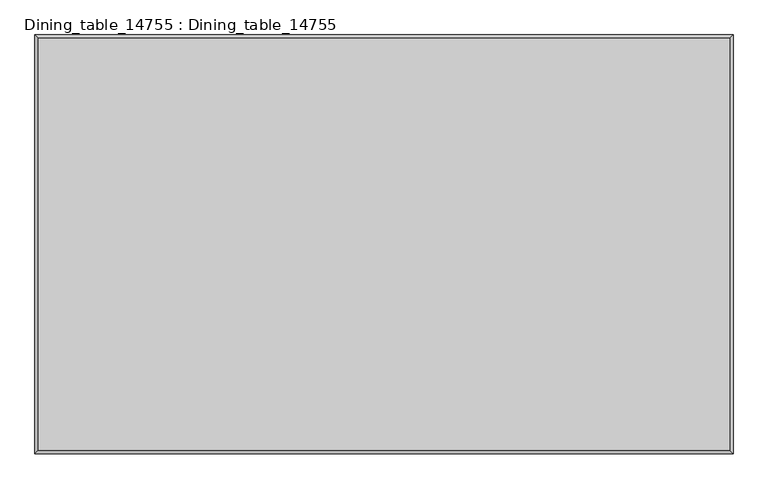
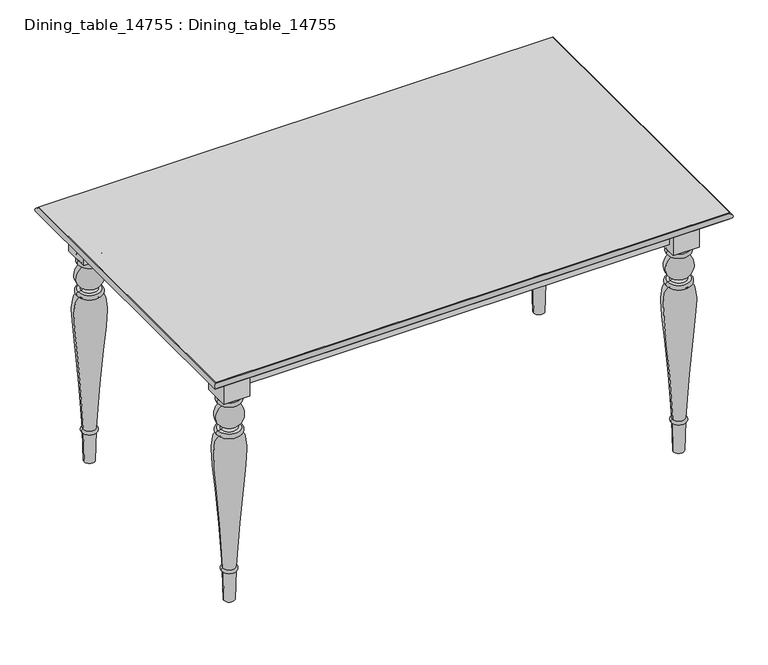
"""IFC4 building model written with IfcOpenShell, lengths in millimetres: furniture geometry, Dining_table_14755 : Dining_table_14755."""

from ifc_helpers import new_model, si_unit, point, frame, origin, place, context, project, spatial, polyline, circle_curve, ellipse_curve, trimmed, outline, extrude, source, transform, mapped, element, save
from ifc_brep_helpers import plane_surface, cylinder_surface, revolved_surface, spline_curve, advanced_brep


def dining_table_14755_dining_table_14755_d89cb775(model_context):
    return source(origin(), model_context, "Body", "SolidModel", [
        extrude(outline(polyline([(137.5044823, 137.5043784), (137.5044823, 62.4956216), (62.4955177, 62.4956216), (62.4955177, 137.5043784), (137.5044823, 137.5043784)])), frame((0.0, 0.0, 630.0), z_axis=(0.0, 0.0, 1.0), x_axis=(1.0, 0.0, 0.0)), (0.0, 0.0, 1.0), 100.0),
        extrude(outline(polyline([(137.5044823, 837.5043784), (137.5044823, 762.4956216), (62.4955177, 762.4956216), (62.4955177, 837.5043784), (137.5044823, 837.5043784)])), frame((0.0, 0.0, 630.0), z_axis=(0.0, 0.0, 1.0), x_axis=(1.0, 0.0, 0.0)), (0.0, 0.0, 1.0), 100.0),
        extrude(outline(polyline([(1437.5044823, 837.5043784), (1437.5044823, 762.4956216), (1362.4955177, 762.4956216), (1362.4955177, 837.5043784), (1437.5044823, 837.5043784)])), frame((0.0, 0.0, 630.0), z_axis=(0.0, 0.0, 1.0), x_axis=(1.0, 0.0, 0.0)), (0.0, 0.0, 1.0), 100.0),
        extrude(outline(polyline([(1437.5044823, 137.5043784), (1437.5044823, 62.4956216), (1362.4955177, 62.4956216), (1362.4955177, 137.5043784), (1437.5044823, 137.5043784)])), frame((0.0, 0.0, 630.0), z_axis=(0.0, 0.0, 1.0), x_axis=(1.0, 0.0, 0.0)), (0.0, 0.0, 1.0), 100.0),
        extrude(outline(polyline([(100.0, 800.0), (100.0, 100.0), (80.0, 100.0), (80.0, 800.0), (100.0, 800.0)])), frame((0.0, 0.0, 655.0), z_axis=(0.0, 0.0, 1.0), x_axis=(1.0, 0.0, 0.0)), (0.0, 0.0, 1.0), 75.0),
        extrude(outline(polyline([(1400.0, 800.0), (100.0, 800.0), (100.0, 820.0), (1400.0, 820.0), (1400.0, 800.0)])), frame((0.0, 0.0, 655.0), z_axis=(0.0, 0.0, 1.0), x_axis=(1.0, 0.0, 0.0)), (0.0, 0.0, 1.0), 75.0),
        extrude(outline(polyline([(1420.0, 800.0), (1420.0, 100.0), (1400.0, 100.0), (1400.0, 800.0), (1420.0, 800.0)])), frame((0.0, 0.0, 655.0), z_axis=(0.0, 0.0, 1.0), x_axis=(1.0, 0.0, 0.0)), (0.0, 0.0, 1.0), 75.0),
        extrude(outline(polyline([(1400.0, 100.0), (1400.0, 80.0), (100.0, 80.0), (100.0, 100.0), (1400.0, 100.0)])), frame((0.0, 0.0, 655.0), z_axis=(0.0, 0.0, 1.0), x_axis=(1.0, 0.0, 0.0)), (0.0, 0.0, 1.0), 75.0),
        advanced_brep(
        [(1492.8253008, 7.1746992, 750.0), (1492.8253008, 892.8253008, 750.0), (7.1746992, 892.8253008, 750.0), (7.1746992, 7.1746992, 750.0), (1492.8253008, 892.8253008, 730.0), (1492.8253008, 7.1746992, 730.0), (7.1746992, 7.1746992, 730.0), (7.1746992, 892.8253008, 730.0), (1492.8253008, 892.8253008, 733.0), (1492.8253008, 7.1746992, 733.0), (1492.8253008, 892.8253008, 747.0), (1492.8253008, 7.1746992, 747.0), (7.1746992, 7.1746992, 733.0), (7.1746992, 7.1746992, 747.0), (7.1746992, 892.8253008, 733.0), (7.1746992, 892.8253008, 747.0)],
        [
            (0, 1),
            (1, 2),
            (2, 3),
            (3, 0),
            (4, 5),
            (5, 6),
            (6, 7),
            (7, 4),
            (8, 9),
            (9, 5),
            (4, 8),
            (8, 10, ellipse_curve(frame((1492.8253008, 892.8253008, 740.0), z_axis=(0.7071067811865475, -0.7071067811865475, 0.0), x_axis=(-0.7071067811865474, -0.7071067811865476, 0.0)), 9.8994949, 7.0)),
            (10, 11),
            (11, 9, ellipse_curve(frame((1492.8253008, 7.1746992, 740.0), z_axis=(0.7071067811865475, 0.7071067811865475, 0.0), x_axis=(0.7071067811865474, -0.7071067811865476, 0.0)), 9.8994949, 7.0)),
            (10, 1),
            (0, 11),
            (9, 12),
            (12, 6),
            (11, 13),
            (13, 12, ellipse_curve(frame((7.1746992, 7.1746992, 740.0), z_axis=(0.7071067811865475, -0.7071067811865475, 0.0), x_axis=(-0.7071067811865476, -0.7071067811865474, 0.0)), 9.8994949, 7.0)),
            (3, 13),
            (12, 14),
            (14, 7),
            (13, 15),
            (15, 14, ellipse_curve(frame((7.1746992, 892.8253008, 740.0), z_axis=(-0.7071067811865475, -0.7071067811865475, 0.0), x_axis=(-0.7071067811865474, 0.7071067811865476, 0.0)), 9.8994949, 7.0)),
            (2, 15),
            (14, 8),
            (15, 10),
        ],
        [
            plane_surface(frame((0.0, 900.0, 750.0), z_axis=(0.0, 0.0, 1.0), x_axis=(-1.0, 0.0, 0.0))),
            plane_surface(frame((0.0, 900.0, 730.0), z_axis=(0.0, 0.0, -1.0), x_axis=(1.0, 0.0, 0.0))),
            plane_surface(frame((1492.8253008, 892.8253008, 730.0), z_axis=(1.0, 0.0, 0.0), x_axis=(0.0, -1.0, 0.0))),
            cylinder_surface(frame((1492.8253008, 900.0, 740.0), z_axis=(0.0, -1.0, 0.0), x_axis=(1.0, 0.0, 0.0)), 7.0),
            plane_surface(frame((1492.8253008, 892.8253008, 747.0), z_axis=(1.0, 0.0, 0.0), x_axis=(0.0, -1.0, 0.0))),
            plane_surface(frame((1492.8253008, 7.1746992, 730.0), z_axis=(0.0, -1.0, 0.0), x_axis=(-1.0, 0.0, 0.0))),
            cylinder_surface(frame((1500.0, 7.1746992, 740.0), z_axis=(-1.0, 0.0, 0.0), x_axis=(0.0, -1.0, 0.0)), 7.0),
            plane_surface(frame((1492.8253008, 7.1746992, 747.0), z_axis=(0.0, -1.0, 0.0), x_axis=(-1.0, 0.0, 0.0))),
            plane_surface(frame((7.1746992, 7.1746992, 730.0), z_axis=(-1.0, 0.0, 0.0), x_axis=(0.0, 1.0, 0.0))),
            cylinder_surface(frame((7.1746992, 0.0, 740.0), z_axis=(0.0, 1.0, 0.0), x_axis=(-1.0, 0.0, 0.0)), 7.0),
            plane_surface(frame((7.1746992, 7.1746992, 747.0), z_axis=(-1.0, 0.0, 0.0), x_axis=(0.0, 1.0, 0.0))),
            plane_surface(frame((7.1746992, 892.8253008, 730.0), z_axis=(0.0, 1.0, 0.0), x_axis=(1.0, 0.0, 0.0))),
            cylinder_surface(frame((0.0, 892.8253008, 740.0), z_axis=(1.0, 0.0, 0.0), x_axis=(0.0, 1.0, 0.0)), 7.0),
            plane_surface(frame((7.1746992, 892.8253008, 747.0), z_axis=(0.0, 1.0, 0.0), x_axis=(1.0, 0.0, 0.0))),
        ],
        [
            (0, [[1, 2, 3, 4]]),
            (1, [[5, 6, 7, 8]]),
            (2, [[9, 10, -5, 11]]),
            (3, [[-9, 12, 13, 14]]),
            (4, [[-13, 15, -1, 16]]),
            (5, [[-10, 17, 18, -6]]),
            (6, [[-14, 19, 20, -17]]),
            (7, [[-16, -4, 21, -19]]),
            (8, [[-18, 22, 23, -7]]),
            (9, [[-20, 24, 25, -22]]),
            (10, [[-21, -3, 26, -24]]),
            (11, [[-11, -8, -23, 27]]),
            (12, [[-12, -27, -25, 28]]),
            (13, [[-15, -28, -26, -2]]),
        ],
    ),
        advanced_brep(
        [(100.0, 100.0, 630.0), (71.6218231, 100.0, 630.0), (128.3781769, 100.0, 630.0), (71.6218231, 100.0, 620.0), (128.3781769, 100.0, 620.0), (71.6218231, 100.0, 607.4843347), (128.3781769, 100.0, 607.4843347), (82.2946134, 100.0, 598.9328748), (117.7053866, 100.0, 598.9328748), (79.4042422, 100.0, 534.8048595), (120.5957578, 100.0, 534.8048595), (77.1750958, 100.0, 526.4855717), (122.8249042, 100.0, 526.4855717), (68.75, 100.0, 525.0), (131.25, 100.0, 525.0), (68.75, 100.0, 513.0), (131.25, 100.0, 513.0), (71.5102534, 100.0, 510.2397466), (128.4897466, 100.0, 510.2397466), (82.3563791, 100.0, 99.9930152), (117.6436209, 100.0, 99.9930152), (82.620575, 100.0, 90.0), (117.379425, 100.0, 90.0), (85.0, 100.0, 0.0), (115.0, 100.0, 0.0), (100.0, 100.0, 0.0)],
        [
            (0, 1),
            (1, 2, circle_curve(frame((100.0, 100.0, 630.0), z_axis=(0.0, 0.0, 1.0), x_axis=(-1.0, 0.0, 0.0)), 28.3781769)),
            (2, 0),
            (2, 1, circle_curve(frame((100.0, 100.0, 630.0), z_axis=(0.0, 0.0, 1.0), x_axis=(-1.0, 0.0, 0.0)), 28.3781769)),
            (1, 3, circle_curve(frame((71.6218231, 100.0, 625.0), z_axis=(0.0, -1.0, 0.0), x_axis=(-1.0, 0.0, 0.0)), 5.0)),
            (3, 4, circle_curve(frame((100.0, 100.0, 620.0), z_axis=(0.0, 0.0, 1.0), x_axis=(-1.0, 0.0, 0.0)), 28.3781769)),
            (4, 2, circle_curve(frame((128.3781769, 100.0, 625.0), z_axis=(0.0, -1.0, 0.0), x_axis=(1.0, 0.0, 0.0)), 5.0)),
            (4, 3, circle_curve(frame((100.0, 100.0, 620.0), z_axis=(0.0, 0.0, 1.0), x_axis=(-1.0, 0.0, 0.0)), 28.3781769)),
            (3, 5, circle_curve(frame((71.6218231, 100.0, 613.7421674), z_axis=(0.0, -1.0, 0.0), x_axis=(-1.0, 0.0, 0.0)), 6.2578326)),
            (5, 6, circle_curve(frame((100.0, 100.0, 607.4843347), z_axis=(0.0, 0.0, 1.0), x_axis=(-1.0, 0.0, 0.0)), 28.3781769)),
            (6, 4, circle_curve(frame((128.3781769, 100.0, 613.7421674), z_axis=(0.0, -1.0, 0.0), x_axis=(1.0, 0.0, 0.0)), 6.2578326)),
            (6, 5, circle_curve(frame((100.0, 100.0, 607.4843347), z_axis=(0.0, 0.0, 1.0), x_axis=(-1.0, 0.0, 0.0)), 28.3781769)),
            (5, 7, circle_curve(frame((71.1386543, 100.0, 595.9454022), z_axis=(0.0, 1.0, 0.0), x_axis=(-1.0, 0.0, 0.0)), 11.5490439)),
            (7, 8, circle_curve(frame((100.0, 100.0, 598.9328748), z_axis=(0.0, 0.0, 1.0), x_axis=(-1.0, 0.0, 0.0)), 17.7053866)),
            (8, 6, circle_curve(frame((128.8613457, 100.0, 595.9454022), z_axis=(0.0, 1.0, 0.0), x_axis=(1.0, 0.0, 0.0)), 11.5490439)),
            (8, 7, circle_curve(frame((100.0, 100.0, 598.9328748), z_axis=(0.0, 0.0, 1.0), x_axis=(-1.0, 0.0, 0.0)), 17.7053866)),
            (7, 9, circle_curve(frame((97.4307139, 100.0, 566.1215172), z_axis=(0.0, -1.0, 0.0), x_axis=(-1.0, 0.0, 0.0)), 36.1342874)),
            (9, 10, circle_curve(frame((100.0, 100.0, 534.8048595), z_axis=(0.0, 0.0, 1.0), x_axis=(-1.0, 0.0, 0.0)), 20.5957578)),
            (10, 8, circle_curve(frame((102.5692861, 100.0, 566.1215172), z_axis=(0.0, -1.0, 0.0), x_axis=(1.0, 0.0, 0.0)), 36.1342874)),
            (10, 9, circle_curve(frame((100.0, 100.0, 534.8048595), z_axis=(0.0, 0.0, 1.0), x_axis=(-1.0, 0.0, 0.0)), 20.5957578)),
            (9, 11, circle_curve(frame((76.3499952, 100.0, 531.1649497), z_axis=(0.0, 1.0, 0.0), x_axis=(-1.0, 0.0, 0.0)), 4.7515649)),
            (11, 12, circle_curve(frame((100.0, 100.0, 526.4855717), z_axis=(0.0, 0.0, 1.0), x_axis=(-1.0, 0.0, 0.0)), 22.8249042)),
            (12, 10, circle_curve(frame((123.6500048, 100.0, 531.1649497), z_axis=(0.0, 1.0, 0.0), x_axis=(1.0, 0.0, 0.0)), 4.7515649)),
            (12, 11, circle_curve(frame((100.0, 100.0, 526.4855717), z_axis=(0.0, 0.0, 1.0), x_axis=(-1.0, 0.0, 0.0)), 22.8249042)),
            (11, 13),
            (13, 14, circle_curve(frame((100.0, 100.0, 525.0), z_axis=(0.0, 0.0, 1.0), x_axis=(-1.0, 0.0, 0.0)), 31.25)),
            (14, 12),
            (14, 13, circle_curve(frame((100.0, 100.0, 525.0), z_axis=(0.0, 0.0, 1.0), x_axis=(-1.0, 0.0, 0.0)), 31.25)),
            (13, 15, circle_curve(frame((68.75, 100.0, 519.0), z_axis=(0.0, -1.0, 0.0), x_axis=(-1.0, 0.0, 0.0)), 6.0)),
            (15, 16, circle_curve(frame((100.0, 100.0, 513.0), z_axis=(0.0, 0.0, 1.0), x_axis=(-1.0, 0.0, 0.0)), 31.25)),
            (16, 14, circle_curve(frame((131.25, 100.0, 519.0), z_axis=(0.0, -1.0, 0.0), x_axis=(1.0, 0.0, 0.0)), 6.0)),
            (16, 15, circle_curve(frame((100.0, 100.0, 513.0), z_axis=(0.0, 0.0, 1.0), x_axis=(-1.0, 0.0, 0.0)), 31.25)),
            (15, 17),
            (17, 18, circle_curve(frame((100.0, 100.0, 510.2397466), z_axis=(0.0, 0.0, 1.0), x_axis=(-1.0, 0.0, 0.0)), 28.4897466)),
            (18, 16),
            (18, 17, circle_curve(frame((100.0, 100.0, 510.2397466), z_axis=(0.0, 0.0, 1.0), x_axis=(-1.0, 0.0, 0.0)), 28.4897466)),
            (17, 19, spline_curve(3, [(71.5102534, 100.0, 510.2397466), (36.079208212, 100.0, 493.717978887), (66.498177461, 100.0, 402.585528177), (82.3563791, 100.0, 99.9930152)], [4, 4], [0.0, 0.4791959451561188])),
            (19, 20, circle_curve(frame((100.0, 100.0, 99.9930152), z_axis=(0.0, 0.0, 1.0), x_axis=(-1.0, 0.0, 0.0)), 17.6436209)),
            (20, 18, spline_curve(3, [(117.6436209, 100.0, 99.9930152), (133.501822539, 100.0, 402.585528177), (163.920791788, 100.0, 493.717978887), (128.4897466, 100.0, 510.2397466)], [4, 4], [0.0, 0.4791959451561188])),
            (20, 19, circle_curve(frame((100.0, 100.0, 99.9930152), z_axis=(0.0, 0.0, 1.0), x_axis=(-1.0, 0.0, 0.0)), 17.6436209)),
            (19, 21, circle_curve(frame((82.620575, 100.0, 95.0), z_axis=(0.0, -1.0, 0.0), x_axis=(-1.0, 0.0, 0.0)), 5.0)),
            (21, 22, circle_curve(frame((100.0, 100.0, 90.0), z_axis=(0.0, 0.0, 1.0), x_axis=(-1.0, 0.0, 0.0)), 17.379425)),
            (22, 20, circle_curve(frame((117.379425, 100.0, 95.0), z_axis=(0.0, -1.0, 0.0), x_axis=(1.0, 0.0, 0.0)), 5.0)),
            (22, 21, circle_curve(frame((100.0, 100.0, 90.0), z_axis=(0.0, 0.0, 1.0), x_axis=(-1.0, 0.0, 0.0)), 17.379425)),
            (21, 23),
            (23, 24, circle_curve(frame((100.0, 100.0, 0.0), z_axis=(0.0, 0.0, 1.0), x_axis=(-1.0, 0.0, 0.0)), 15.0)),
            (24, 22),
            (24, 23, circle_curve(frame((100.0, 100.0, 0.0), z_axis=(0.0, 0.0, 1.0), x_axis=(-1.0, 0.0, 0.0)), 15.0)),
            (23, 25),
            (25, 24),
        ],
        [
            plane_surface(frame((100.0, 100.0, 630.0), z_axis=(0.0, 0.0, 1.0), x_axis=(-1.0, 0.0, 0.0))),
            revolved_surface(trimmed(ellipse_curve(frame((71.6218231, 100.0, 625.0), z_axis=(0.0, 1.0, 0.0), x_axis=(-1.0, 0.0, 0.0)), 5.0, 5.0), [point((71.6218231, 100.0, 620.0))], [point((71.6218231, 100.0, 630.0))], True, "CARTESIAN"), (100.0, 100.0, 950.0), (0.0, 0.0, 1.0)),
            revolved_surface(trimmed(ellipse_curve(frame((71.6218231, 100.0, 613.7421674), z_axis=(0.0, 1.0, 0.0), x_axis=(-1.0, 0.0, 0.0)), 6.2578326, 6.2578326), [point((71.6218231, 100.0, 607.4843347))], [point((71.6218231, 100.0, 620.0))], True, "CARTESIAN"), (100.0, 100.0, 950.0), (0.0, 0.0, 1.0)),
            revolved_surface(trimmed(ellipse_curve(frame((71.1386543, 100.0, 595.9454022), z_axis=(0.0, -1.0, 0.0), x_axis=(-1.0, 0.0, 0.0)), 11.5490439, 11.5490439), [point((82.2946134, 100.0, 598.9328748))], [point((71.6218231, 100.0, 607.4843347))], True, "CARTESIAN"), (100.0, 100.0, 950.0), (0.0, 0.0, 1.0)),
            revolved_surface(trimmed(ellipse_curve(frame((97.4307139, 100.0, 566.1215172), z_axis=(0.0, 1.0, 0.0), x_axis=(-1.0, 0.0, 0.0)), 36.1342874, 36.1342874), [point((79.4042422, 100.0, 534.8048595))], [point((82.2946134, 100.0, 598.9328748))], True, "CARTESIAN"), (100.0, 100.0, 950.0), (0.0, 0.0, 1.0)),
            revolved_surface(trimmed(ellipse_curve(frame((76.3499952, 100.0, 531.1649497), z_axis=(0.0, -1.0, 0.0), x_axis=(-1.0, 0.0, 0.0)), 4.7515649, 4.7515649), [point((77.1750958, 100.0, 526.4855717))], [point((79.4042422, 100.0, 534.8048595))], True, "CARTESIAN"), (100.0, 100.0, 950.0), (0.0, 0.0, 1.0)),
            revolved_surface(polyline([(68.75, 100.0, 525.0), (77.1750958, 100.0, 526.4855717)]), (100.0, 100.0, 950.0), (0.0, 0.0, 1.0)),
            revolved_surface(trimmed(ellipse_curve(frame((68.75, 100.0, 519.0), z_axis=(0.0, 1.0, 0.0), x_axis=(-1.0, 0.0, 0.0)), 6.0, 6.0), [point((68.75, 100.0, 513.0))], [point((68.75, 100.0, 525.0))], True, "CARTESIAN"), (100.0, 100.0, 950.0), (0.0, 0.0, 1.0)),
            revolved_surface(polyline([(71.5102534, 100.0, 510.2397466), (68.75, 100.0, 513.0)]), (100.0, 100.0, 950.0), (0.0, 0.0, 1.0)),
            revolved_surface(spline_curve(3, [(82.3563791, 100.0, 99.9930152), (66.498177461, 100.0, 402.585528177), (36.079208212, 100.0, 493.717978887), (71.5102534, 100.0, 510.2397466)], [4, 4], [0.0, 0.4791959451561188]), (100.0, 100.0, 950.0), (0.0, 0.0, 1.0)),
            revolved_surface(trimmed(ellipse_curve(frame((82.620575, 100.0, 95.0), z_axis=(0.0, 1.0, 0.0), x_axis=(-1.0, 0.0, 0.0)), 5.0, 5.0), [point((82.620575, 100.0, 90.0))], [point((82.3563791, 100.0, 99.9930152))], True, "CARTESIAN"), (100.0, 100.0, 950.0), (0.0, 0.0, 1.0)),
            revolved_surface(polyline([(85.0, 100.0, 0.0), (82.620575, 100.0, 90.0)]), (100.0, 100.0, 950.0), (0.0, 0.0, 1.0)),
            plane_surface(frame((100.0, 100.0, 0.0), z_axis=(0.0, 0.0, -1.0), x_axis=(-1.0, 0.0, 0.0))),
        ],
        [
            (0, [[1, 2, 3]]),
            (0, [[-3, 4, -1]]),
            (1, [[-2, 5, 6, 7]]),
            (1, [[-4, -7, 8, -5]]),
            (2, [[-6, 9, 10, 11]]),
            (2, [[-8, -11, 12, -9]]),
            (3, [[-10, 13, 14, 15]]),
            (3, [[-12, -15, 16, -13]]),
            (4, [[-14, 17, 18, 19]]),
            (4, [[-16, -19, 20, -17]]),
            (5, [[-18, 21, 22, 23]]),
            (5, [[-20, -23, 24, -21]]),
            (6, [[-22, 25, 26, 27]]),
            (6, [[-24, -27, 28, -25]]),
            (7, [[-26, 29, 30, 31]]),
            (7, [[-28, -31, 32, -29]]),
            (8, [[-30, 33, 34, 35]]),
            (8, [[-32, -35, 36, -33]]),
            (9, [[-34, 37, 38, 39]]),
            (9, [[-36, -39, 40, -37]]),
            (10, [[-38, 41, 42, 43]]),
            (10, [[-40, -43, 44, -41]]),
            (11, [[-42, 45, 46, 47]]),
            (11, [[-44, -47, 48, -45]]),
            (12, [[-46, 49, 50]]),
            (12, [[-48, -50, -49]]),
        ],
    ),
        advanced_brep(
        [(100.0, 800.0, 630.0), (71.6218231, 800.0, 630.0), (128.3781769, 800.0, 630.0), (71.6218231, 800.0, 620.0), (128.3781769, 800.0, 620.0), (71.6218231, 800.0, 607.4843347), (128.3781769, 800.0, 607.4843347), (82.2946134, 800.0, 598.9328748), (117.7053866, 800.0, 598.9328748), (79.4042422, 800.0, 534.8048595), (120.5957578, 800.0, 534.8048595), (77.1750958, 800.0, 526.4855717), (122.8249042, 800.0, 526.4855717), (68.75, 800.0, 525.0), (131.25, 800.0, 525.0), (68.75, 800.0, 513.0), (131.25, 800.0, 513.0), (71.5102534, 800.0, 510.2397466), (128.4897466, 800.0, 510.2397466), (82.3563791, 800.0, 99.9930152), (117.6436209, 800.0, 99.9930152), (82.620575, 800.0, 90.0), (117.379425, 800.0, 90.0), (85.0, 800.0, 0.0), (115.0, 800.0, 0.0), (100.0, 800.0, 0.0)],
        [
            (0, 1),
            (1, 2, circle_curve(frame((100.0, 800.0, 630.0), z_axis=(0.0, 0.0, 1.0), x_axis=(-1.0, 0.0, 0.0)), 28.3781769)),
            (2, 0),
            (2, 1, circle_curve(frame((100.0, 800.0, 630.0), z_axis=(0.0, 0.0, 1.0), x_axis=(-1.0, 0.0, 0.0)), 28.3781769)),
            (1, 3, circle_curve(frame((71.6218231, 800.0, 625.0), z_axis=(0.0, -1.0, 0.0), x_axis=(-1.0, 0.0, 0.0)), 5.0)),
            (3, 4, circle_curve(frame((100.0, 800.0, 620.0), z_axis=(0.0, 0.0, 1.0), x_axis=(-1.0, 0.0, 0.0)), 28.3781769)),
            (4, 2, circle_curve(frame((128.3781769, 800.0, 625.0), z_axis=(0.0, -1.0, 0.0), x_axis=(1.0, 0.0, 0.0)), 5.0)),
            (4, 3, circle_curve(frame((100.0, 800.0, 620.0), z_axis=(0.0, 0.0, 1.0), x_axis=(-1.0, 0.0, 0.0)), 28.3781769)),
            (3, 5, circle_curve(frame((71.6218231, 800.0, 613.7421674), z_axis=(0.0, -1.0, 0.0), x_axis=(-1.0, 0.0, 0.0)), 6.2578326)),
            (5, 6, circle_curve(frame((100.0, 800.0, 607.4843347), z_axis=(0.0, 0.0, 1.0), x_axis=(-1.0, 0.0, 0.0)), 28.3781769)),
            (6, 4, circle_curve(frame((128.3781769, 800.0, 613.7421674), z_axis=(0.0, -1.0, 0.0), x_axis=(1.0, 0.0, 0.0)), 6.2578326)),
            (6, 5, circle_curve(frame((100.0, 800.0, 607.4843347), z_axis=(0.0, 0.0, 1.0), x_axis=(-1.0, 0.0, 0.0)), 28.3781769)),
            (5, 7, circle_curve(frame((71.1386543, 800.0, 595.9454022), z_axis=(0.0, 1.0, 0.0), x_axis=(-1.0, 0.0, 0.0)), 11.5490439)),
            (7, 8, circle_curve(frame((100.0, 800.0, 598.9328748), z_axis=(0.0, 0.0, 1.0), x_axis=(-1.0, 0.0, 0.0)), 17.7053866)),
            (8, 6, circle_curve(frame((128.8613457, 800.0, 595.9454022), z_axis=(0.0, 1.0, 0.0), x_axis=(1.0, 0.0, 0.0)), 11.5490439)),
            (8, 7, circle_curve(frame((100.0, 800.0, 598.9328748), z_axis=(0.0, 0.0, 1.0), x_axis=(-1.0, 0.0, 0.0)), 17.7053866)),
            (7, 9, circle_curve(frame((97.4307139, 800.0, 566.1215172), z_axis=(0.0, -1.0, 0.0), x_axis=(-1.0, 0.0, 0.0)), 36.1342874)),
            (9, 10, circle_curve(frame((100.0, 800.0, 534.8048595), z_axis=(0.0, 0.0, 1.0), x_axis=(-1.0, 0.0, 0.0)), 20.5957578)),
            (10, 8, circle_curve(frame((102.5692861, 800.0, 566.1215172), z_axis=(0.0, -1.0, 0.0), x_axis=(1.0, 0.0, 0.0)), 36.1342874)),
            (10, 9, circle_curve(frame((100.0, 800.0, 534.8048595), z_axis=(0.0, 0.0, 1.0), x_axis=(-1.0, 0.0, 0.0)), 20.5957578)),
            (9, 11, circle_curve(frame((76.3499952, 800.0, 531.1649497), z_axis=(0.0, 1.0, 0.0), x_axis=(-1.0, 0.0, 0.0)), 4.7515649)),
            (11, 12, circle_curve(frame((100.0, 800.0, 526.4855717), z_axis=(0.0, 0.0, 1.0), x_axis=(-1.0, 0.0, 0.0)), 22.8249042)),
            (12, 10, circle_curve(frame((123.6500048, 800.0, 531.1649497), z_axis=(0.0, 1.0, 0.0), x_axis=(1.0, 0.0, 0.0)), 4.7515649)),
            (12, 11, circle_curve(frame((100.0, 800.0, 526.4855717), z_axis=(0.0, 0.0, 1.0), x_axis=(-1.0, 0.0, 0.0)), 22.8249042)),
            (11, 13),
            (13, 14, circle_curve(frame((100.0, 800.0, 525.0), z_axis=(0.0, 0.0, 1.0), x_axis=(-1.0, 0.0, 0.0)), 31.25)),
            (14, 12),
            (14, 13, circle_curve(frame((100.0, 800.0, 525.0), z_axis=(0.0, 0.0, 1.0), x_axis=(-1.0, 0.0, 0.0)), 31.25)),
            (13, 15, circle_curve(frame((68.75, 800.0, 519.0), z_axis=(0.0, -1.0, 0.0), x_axis=(-1.0, 0.0, 0.0)), 6.0)),
            (15, 16, circle_curve(frame((100.0, 800.0, 513.0), z_axis=(0.0, 0.0, 1.0), x_axis=(-1.0, 0.0, 0.0)), 31.25)),
            (16, 14, circle_curve(frame((131.25, 800.0, 519.0), z_axis=(0.0, -1.0, 0.0), x_axis=(1.0, 0.0, 0.0)), 6.0)),
            (16, 15, circle_curve(frame((100.0, 800.0, 513.0), z_axis=(0.0, 0.0, 1.0), x_axis=(-1.0, 0.0, 0.0)), 31.25)),
            (15, 17),
            (17, 18, circle_curve(frame((100.0, 800.0, 510.2397466), z_axis=(0.0, 0.0, 1.0), x_axis=(-1.0, 0.0, 0.0)), 28.4897466)),
            (18, 16),
            (18, 17, circle_curve(frame((100.0, 800.0, 510.2397466), z_axis=(0.0, 0.0, 1.0), x_axis=(-1.0, 0.0, 0.0)), 28.4897466)),
            (17, 19, spline_curve(3, [(71.5102534, 800.0, 510.2397466), (36.079208212, 800.0, 493.717978887), (66.498177461, 800.0, 402.585528177), (82.3563791, 800.0, 99.9930152)], [4, 4], [0.0, 0.4791959451561188])),
            (19, 20, circle_curve(frame((100.0, 800.0, 99.9930152), z_axis=(0.0, 0.0, 1.0), x_axis=(-1.0, 0.0, 0.0)), 17.6436209)),
            (20, 18, spline_curve(3, [(117.6436209, 800.0, 99.9930152), (133.501822539, 800.0, 402.585528177), (163.920791788, 800.0, 493.717978887), (128.4897466, 800.0, 510.2397466)], [4, 4], [0.0, 0.4791959451561188])),
            (20, 19, circle_curve(frame((100.0, 800.0, 99.9930152), z_axis=(0.0, 0.0, 1.0), x_axis=(-1.0, 0.0, 0.0)), 17.6436209)),
            (19, 21, circle_curve(frame((82.620575, 800.0, 95.0), z_axis=(0.0, -1.0, 0.0), x_axis=(-1.0, 0.0, 0.0)), 5.0)),
            (21, 22, circle_curve(frame((100.0, 800.0, 90.0), z_axis=(0.0, 0.0, 1.0), x_axis=(-1.0, 0.0, 0.0)), 17.379425)),
            (22, 20, circle_curve(frame((117.379425, 800.0, 95.0), z_axis=(0.0, -1.0, 0.0), x_axis=(1.0, 0.0, 0.0)), 5.0)),
            (22, 21, circle_curve(frame((100.0, 800.0, 90.0), z_axis=(0.0, 0.0, 1.0), x_axis=(-1.0, 0.0, 0.0)), 17.379425)),
            (21, 23),
            (23, 24, circle_curve(frame((100.0, 800.0, 0.0), z_axis=(0.0, 0.0, 1.0), x_axis=(-1.0, 0.0, 0.0)), 15.0)),
            (24, 22),
            (24, 23, circle_curve(frame((100.0, 800.0, 0.0), z_axis=(0.0, 0.0, 1.0), x_axis=(-1.0, 0.0, 0.0)), 15.0)),
            (23, 25),
            (25, 24),
        ],
        [
            plane_surface(frame((100.0, 800.0, 630.0), z_axis=(0.0, 0.0, 1.0), x_axis=(-1.0, 0.0, 0.0))),
            revolved_surface(trimmed(ellipse_curve(frame((71.6218231, 800.0, 625.0), z_axis=(0.0, 1.0, 0.0), x_axis=(-1.0, 0.0, 0.0)), 5.0, 5.0), [point((71.6218231, 800.0, 620.0))], [point((71.6218231, 800.0, 630.0))], True, "CARTESIAN"), (100.0, 800.0, 950.0), (0.0, 0.0, 1.0)),
            revolved_surface(trimmed(ellipse_curve(frame((71.6218231, 800.0, 613.7421674), z_axis=(0.0, 1.0, 0.0), x_axis=(-1.0, 0.0, 0.0)), 6.2578326, 6.2578326), [point((71.6218231, 800.0, 607.4843347))], [point((71.6218231, 800.0, 620.0))], True, "CARTESIAN"), (100.0, 800.0, 950.0), (0.0, 0.0, 1.0)),
            revolved_surface(trimmed(ellipse_curve(frame((71.1386543, 800.0, 595.9454022), z_axis=(0.0, -1.0, 0.0), x_axis=(-1.0, 0.0, 0.0)), 11.5490439, 11.5490439), [point((82.2946134, 800.0, 598.9328748))], [point((71.6218231, 800.0, 607.4843347))], True, "CARTESIAN"), (100.0, 800.0, 950.0), (0.0, 0.0, 1.0)),
            revolved_surface(trimmed(ellipse_curve(frame((97.4307139, 800.0, 566.1215172), z_axis=(0.0, 1.0, 0.0), x_axis=(-1.0, 0.0, 0.0)), 36.1342874, 36.1342874), [point((79.4042422, 800.0, 534.8048595))], [point((82.2946134, 800.0, 598.9328748))], True, "CARTESIAN"), (100.0, 800.0, 950.0), (0.0, 0.0, 1.0)),
            revolved_surface(trimmed(ellipse_curve(frame((76.3499952, 800.0, 531.1649497), z_axis=(0.0, -1.0, 0.0), x_axis=(-1.0, 0.0, 0.0)), 4.7515649, 4.7515649), [point((77.1750958, 800.0, 526.4855717))], [point((79.4042422, 800.0, 534.8048595))], True, "CARTESIAN"), (100.0, 800.0, 950.0), (0.0, 0.0, 1.0)),
            revolved_surface(polyline([(68.75, 800.0, 525.0), (77.1750958, 800.0, 526.4855717)]), (100.0, 800.0, 950.0), (0.0, 0.0, 1.0)),
            revolved_surface(trimmed(ellipse_curve(frame((68.75, 800.0, 519.0), z_axis=(0.0, 1.0, 0.0), x_axis=(-1.0, 0.0, 0.0)), 6.0, 6.0), [point((68.75, 800.0, 513.0))], [point((68.75, 800.0, 525.0))], True, "CARTESIAN"), (100.0, 800.0, 950.0), (0.0, 0.0, 1.0)),
            revolved_surface(polyline([(71.5102534, 800.0, 510.2397466), (68.75, 800.0, 513.0)]), (100.0, 800.0, 950.0), (0.0, 0.0, 1.0)),
            revolved_surface(spline_curve(3, [(82.3563791, 800.0, 99.9930152), (66.498177461, 800.0, 402.585528177), (36.079208212, 800.0, 493.717978887), (71.5102534, 800.0, 510.2397466)], [4, 4], [0.0, 0.4791959451561188]), (100.0, 800.0, 950.0), (0.0, 0.0, 1.0)),
            revolved_surface(trimmed(ellipse_curve(frame((82.620575, 800.0, 95.0), z_axis=(0.0, 1.0, 0.0), x_axis=(-1.0, 0.0, 0.0)), 5.0, 5.0), [point((82.620575, 800.0, 90.0))], [point((82.3563791, 800.0, 99.9930152))], True, "CARTESIAN"), (100.0, 800.0, 950.0), (0.0, 0.0, 1.0)),
            revolved_surface(polyline([(85.0, 800.0, 0.0), (82.620575, 800.0, 90.0)]), (100.0, 800.0, 950.0), (0.0, 0.0, 1.0)),
            plane_surface(frame((100.0, 800.0, 0.0), z_axis=(0.0, 0.0, -1.0), x_axis=(-1.0, 0.0, 0.0))),
        ],
        [
            (0, [[1, 2, 3]]),
            (0, [[-3, 4, -1]]),
            (1, [[-2, 5, 6, 7]]),
            (1, [[-4, -7, 8, -5]]),
            (2, [[-6, 9, 10, 11]]),
            (2, [[-8, -11, 12, -9]]),
            (3, [[-10, 13, 14, 15]]),
            (3, [[-12, -15, 16, -13]]),
            (4, [[-14, 17, 18, 19]]),
            (4, [[-16, -19, 20, -17]]),
            (5, [[-18, 21, 22, 23]]),
            (5, [[-20, -23, 24, -21]]),
            (6, [[-22, 25, 26, 27]]),
            (6, [[-24, -27, 28, -25]]),
            (7, [[-26, 29, 30, 31]]),
            (7, [[-28, -31, 32, -29]]),
            (8, [[-30, 33, 34, 35]]),
            (8, [[-32, -35, 36, -33]]),
            (9, [[-34, 37, 38, 39]]),
            (9, [[-36, -39, 40, -37]]),
            (10, [[-38, 41, 42, 43]]),
            (10, [[-40, -43, 44, -41]]),
            (11, [[-42, 45, 46, 47]]),
            (11, [[-44, -47, 48, -45]]),
            (12, [[-46, 49, 50]]),
            (12, [[-48, -50, -49]]),
        ],
    ),
        advanced_brep(
        [(1400.0, 800.0, 630.0), (1371.6218231, 800.0, 630.0), (1428.3781769, 800.0, 630.0), (1371.6218231, 800.0, 620.0), (1428.3781769, 800.0, 620.0), (1371.6218231, 800.0, 607.4843347), (1428.3781769, 800.0, 607.4843347), (1382.2946134, 800.0, 598.9328748), (1417.7053866, 800.0, 598.9328748), (1379.4042422, 800.0, 534.8048595), (1420.5957578, 800.0, 534.8048595), (1377.1750958, 800.0, 526.4855717), (1422.8249042, 800.0, 526.4855717), (1368.75, 800.0, 525.0), (1431.25, 800.0, 525.0), (1368.75, 800.0, 513.0), (1431.25, 800.0, 513.0), (1371.5102534, 800.0, 510.2397466), (1428.4897466, 800.0, 510.2397466), (1382.3563791, 800.0, 99.9930152), (1417.6436209, 800.0, 99.9930152), (1382.620575, 800.0, 90.0), (1417.379425, 800.0, 90.0), (1385.0, 800.0, 0.0), (1415.0, 800.0, 0.0), (1400.0, 800.0, 0.0)],
        [
            (0, 1),
            (1, 2, circle_curve(frame((1400.0, 800.0, 630.0), z_axis=(0.0, 0.0, 1.0), x_axis=(-1.0, 0.0, 0.0)), 28.3781769)),
            (2, 0),
            (2, 1, circle_curve(frame((1400.0, 800.0, 630.0), z_axis=(0.0, 0.0, 1.0), x_axis=(-1.0, 0.0, 0.0)), 28.3781769)),
            (1, 3, circle_curve(frame((1371.6218231, 800.0, 625.0), z_axis=(0.0, -1.0, 0.0), x_axis=(-1.0, 0.0, 0.0)), 5.0)),
            (3, 4, circle_curve(frame((1400.0, 800.0, 620.0), z_axis=(0.0, 0.0, 1.0), x_axis=(-1.0, 0.0, 0.0)), 28.3781769)),
            (4, 2, circle_curve(frame((1428.3781769, 800.0, 625.0), z_axis=(0.0, -1.0, 0.0), x_axis=(1.0, 0.0, 0.0)), 5.0)),
            (4, 3, circle_curve(frame((1400.0, 800.0, 620.0), z_axis=(0.0, 0.0, 1.0), x_axis=(-1.0, 0.0, 0.0)), 28.3781769)),
            (3, 5, circle_curve(frame((1371.6218231, 800.0, 613.7421674), z_axis=(0.0, -1.0, 0.0), x_axis=(-1.0, 0.0, 0.0)), 6.2578326)),
            (5, 6, circle_curve(frame((1400.0, 800.0, 607.4843347), z_axis=(0.0, 0.0, 1.0), x_axis=(-1.0, 0.0, 0.0)), 28.3781769)),
            (6, 4, circle_curve(frame((1428.3781769, 800.0, 613.7421674), z_axis=(0.0, -1.0, 0.0), x_axis=(1.0, 0.0, 0.0)), 6.2578326)),
            (6, 5, circle_curve(frame((1400.0, 800.0, 607.4843347), z_axis=(0.0, 0.0, 1.0), x_axis=(-1.0, 0.0, 0.0)), 28.3781769)),
            (5, 7, circle_curve(frame((1371.1386543, 800.0, 595.9454022), z_axis=(0.0, 1.0, 0.0), x_axis=(-1.0, 0.0, 0.0)), 11.5490439)),
            (7, 8, circle_curve(frame((1400.0, 800.0, 598.9328748), z_axis=(0.0, 0.0, 1.0), x_axis=(-1.0, 0.0, 0.0)), 17.7053866)),
            (8, 6, circle_curve(frame((1428.8613457, 800.0, 595.9454022), z_axis=(0.0, 1.0, 0.0), x_axis=(1.0, 0.0, 0.0)), 11.5490439)),
            (8, 7, circle_curve(frame((1400.0, 800.0, 598.9328748), z_axis=(0.0, 0.0, 1.0), x_axis=(-1.0, 0.0, 0.0)), 17.7053866)),
            (7, 9, circle_curve(frame((1397.4307139, 800.0, 566.1215172), z_axis=(0.0, -1.0, 0.0), x_axis=(-1.0, 0.0, 0.0)), 36.1342874)),
            (9, 10, circle_curve(frame((1400.0, 800.0, 534.8048595), z_axis=(0.0, 0.0, 1.0), x_axis=(-1.0, 0.0, 0.0)), 20.5957578)),
            (10, 8, circle_curve(frame((1402.5692861, 800.0, 566.1215172), z_axis=(0.0, -1.0, 0.0), x_axis=(1.0, 0.0, 0.0)), 36.1342874)),
            (10, 9, circle_curve(frame((1400.0, 800.0, 534.8048595), z_axis=(0.0, 0.0, 1.0), x_axis=(-1.0, 0.0, 0.0)), 20.5957578)),
            (9, 11, circle_curve(frame((1376.3499952, 800.0, 531.1649497), z_axis=(0.0, 1.0, 0.0), x_axis=(-1.0, 0.0, 0.0)), 4.7515649)),
            (11, 12, circle_curve(frame((1400.0, 800.0, 526.4855717), z_axis=(0.0, 0.0, 1.0), x_axis=(-1.0, 0.0, 0.0)), 22.8249042)),
            (12, 10, circle_curve(frame((1423.6500048, 800.0, 531.1649497), z_axis=(0.0, 1.0, 0.0), x_axis=(1.0, 0.0, 0.0)), 4.7515649)),
            (12, 11, circle_curve(frame((1400.0, 800.0, 526.4855717), z_axis=(0.0, 0.0, 1.0), x_axis=(-1.0, 0.0, 0.0)), 22.8249042)),
            (11, 13),
            (13, 14, circle_curve(frame((1400.0, 800.0, 525.0), z_axis=(0.0, 0.0, 1.0), x_axis=(-1.0, 0.0, 0.0)), 31.25)),
            (14, 12),
            (14, 13, circle_curve(frame((1400.0, 800.0, 525.0), z_axis=(0.0, 0.0, 1.0), x_axis=(-1.0, 0.0, 0.0)), 31.25)),
            (13, 15, circle_curve(frame((1368.75, 800.0, 519.0), z_axis=(0.0, -1.0, 0.0), x_axis=(-1.0, 0.0, 0.0)), 6.0)),
            (15, 16, circle_curve(frame((1400.0, 800.0, 513.0), z_axis=(0.0, 0.0, 1.0), x_axis=(-1.0, 0.0, 0.0)), 31.25)),
            (16, 14, circle_curve(frame((1431.25, 800.0, 519.0), z_axis=(0.0, -1.0, 0.0), x_axis=(1.0, 0.0, 0.0)), 6.0)),
            (16, 15, circle_curve(frame((1400.0, 800.0, 513.0), z_axis=(0.0, 0.0, 1.0), x_axis=(-1.0, 0.0, 0.0)), 31.25)),
            (15, 17),
            (17, 18, circle_curve(frame((1400.0, 800.0, 510.2397466), z_axis=(0.0, 0.0, 1.0), x_axis=(-1.0, 0.0, 0.0)), 28.4897466)),
            (18, 16),
            (18, 17, circle_curve(frame((1400.0, 800.0, 510.2397466), z_axis=(0.0, 0.0, 1.0), x_axis=(-1.0, 0.0, 0.0)), 28.4897466)),
            (17, 19, spline_curve(3, [(1371.5102534, 800.0, 510.2397466), (1336.079208212, 800.0, 493.717978887), (1366.498177461, 800.0, 402.585528177), (1382.3563791, 800.0, 99.9930152)], [4, 4], [0.0, 0.4791959451561188])),
            (19, 20, circle_curve(frame((1400.0, 800.0, 99.9930152), z_axis=(0.0, 0.0, 1.0), x_axis=(-1.0, 0.0, 0.0)), 17.6436209)),
            (20, 18, spline_curve(3, [(1417.6436209, 800.0, 99.9930152), (1433.501822539, 800.0, 402.585528177), (1463.920791788, 800.0, 493.717978887), (1428.4897466, 800.0, 510.2397466)], [4, 4], [0.0, 0.4791959451561188])),
            (20, 19, circle_curve(frame((1400.0, 800.0, 99.9930152), z_axis=(0.0, 0.0, 1.0), x_axis=(-1.0, 0.0, 0.0)), 17.6436209)),
            (19, 21, circle_curve(frame((1382.620575, 800.0, 95.0), z_axis=(0.0, -1.0, 0.0), x_axis=(-1.0, 0.0, 0.0)), 5.0)),
            (21, 22, circle_curve(frame((1400.0, 800.0, 90.0), z_axis=(0.0, 0.0, 1.0), x_axis=(-1.0, 0.0, 0.0)), 17.379425)),
            (22, 20, circle_curve(frame((1417.379425, 800.0, 95.0), z_axis=(0.0, -1.0, 0.0), x_axis=(1.0, 0.0, 0.0)), 5.0)),
            (22, 21, circle_curve(frame((1400.0, 800.0, 90.0), z_axis=(0.0, 0.0, 1.0), x_axis=(-1.0, 0.0, 0.0)), 17.379425)),
            (21, 23),
            (23, 24, circle_curve(frame((1400.0, 800.0, 0.0), z_axis=(0.0, 0.0, 1.0), x_axis=(-1.0, 0.0, 0.0)), 15.0)),
            (24, 22),
            (24, 23, circle_curve(frame((1400.0, 800.0, 0.0), z_axis=(0.0, 0.0, 1.0), x_axis=(-1.0, 0.0, 0.0)), 15.0)),
            (23, 25),
            (25, 24),
        ],
        [
            plane_surface(frame((1400.0, 800.0, 630.0), z_axis=(0.0, 0.0, 1.0), x_axis=(-1.0, 0.0, 0.0))),
            revolved_surface(trimmed(ellipse_curve(frame((1371.6218231, 800.0, 625.0), z_axis=(0.0, 1.0, 0.0), x_axis=(-1.0, 0.0, 0.0)), 5.0, 5.0), [point((1371.6218231, 800.0, 620.0))], [point((1371.6218231, 800.0, 630.0))], True, "CARTESIAN"), (1400.0, 800.0, 950.0), (0.0, 0.0, 1.0)),
            revolved_surface(trimmed(ellipse_curve(frame((1371.6218231, 800.0, 613.7421674), z_axis=(0.0, 1.0, 0.0), x_axis=(-1.0, 0.0, 0.0)), 6.2578326, 6.2578326), [point((1371.6218231, 800.0, 607.4843347))], [point((1371.6218231, 800.0, 620.0))], True, "CARTESIAN"), (1400.0, 800.0, 950.0), (0.0, 0.0, 1.0)),
            revolved_surface(trimmed(ellipse_curve(frame((1371.1386543, 800.0, 595.9454022), z_axis=(0.0, -1.0, 0.0), x_axis=(-1.0, 0.0, 0.0)), 11.5490439, 11.5490439), [point((1382.2946134, 800.0, 598.9328748))], [point((1371.6218231, 800.0, 607.4843347))], True, "CARTESIAN"), (1400.0, 800.0, 950.0), (0.0, 0.0, 1.0)),
            revolved_surface(trimmed(ellipse_curve(frame((1397.4307139, 800.0, 566.1215172), z_axis=(0.0, 1.0, 0.0), x_axis=(-1.0, 0.0, 0.0)), 36.1342874, 36.1342874), [point((1379.4042422, 800.0, 534.8048595))], [point((1382.2946134, 800.0, 598.9328748))], True, "CARTESIAN"), (1400.0, 800.0, 950.0), (0.0, 0.0, 1.0)),
            revolved_surface(trimmed(ellipse_curve(frame((1376.3499952, 800.0, 531.1649497), z_axis=(0.0, -1.0, 0.0), x_axis=(-1.0, 0.0, 0.0)), 4.7515649, 4.7515649), [point((1377.1750958, 800.0, 526.4855717))], [point((1379.4042422, 800.0, 534.8048595))], True, "CARTESIAN"), (1400.0, 800.0, 950.0), (0.0, 0.0, 1.0)),
            revolved_surface(polyline([(1368.75, 800.0, 525.0), (1377.1750958, 800.0, 526.4855717)]), (1400.0, 800.0, 950.0), (0.0, 0.0, 1.0)),
            revolved_surface(trimmed(ellipse_curve(frame((1368.75, 800.0, 519.0), z_axis=(0.0, 1.0, 0.0), x_axis=(-1.0, 0.0, 0.0)), 6.0, 6.0), [point((1368.75, 800.0, 513.0))], [point((1368.75, 800.0, 525.0))], True, "CARTESIAN"), (1400.0, 800.0, 950.0), (0.0, 0.0, 1.0)),
            revolved_surface(polyline([(1371.5102534, 800.0, 510.2397466), (1368.75, 800.0, 513.0)]), (1400.0, 800.0, 950.0), (0.0, 0.0, 1.0)),
            revolved_surface(spline_curve(3, [(1382.3563791, 800.0, 99.9930152), (1366.498177461, 800.0, 402.585528177), (1336.079208212, 800.0, 493.717978887), (1371.5102534, 800.0, 510.2397466)], [4, 4], [0.0, 0.4791959451561188]), (1400.0, 800.0, 950.0), (0.0, 0.0, 1.0)),
            revolved_surface(trimmed(ellipse_curve(frame((1382.620575, 800.0, 95.0), z_axis=(0.0, 1.0, 0.0), x_axis=(-1.0, 0.0, 0.0)), 5.0, 5.0), [point((1382.620575, 800.0, 90.0))], [point((1382.3563791, 800.0, 99.9930152))], True, "CARTESIAN"), (1400.0, 800.0, 950.0), (0.0, 0.0, 1.0)),
            revolved_surface(polyline([(1385.0, 800.0, 0.0), (1382.620575, 800.0, 90.0)]), (1400.0, 800.0, 950.0), (0.0, 0.0, 1.0)),
            plane_surface(frame((1400.0, 800.0, 0.0), z_axis=(0.0, 0.0, -1.0), x_axis=(-1.0, 0.0, 0.0))),
        ],
        [
            (0, [[1, 2, 3]]),
            (0, [[-3, 4, -1]]),
            (1, [[-2, 5, 6, 7]]),
            (1, [[-4, -7, 8, -5]]),
            (2, [[-6, 9, 10, 11]]),
            (2, [[-8, -11, 12, -9]]),
            (3, [[-10, 13, 14, 15]]),
            (3, [[-12, -15, 16, -13]]),
            (4, [[-14, 17, 18, 19]]),
            (4, [[-16, -19, 20, -17]]),
            (5, [[-18, 21, 22, 23]]),
            (5, [[-20, -23, 24, -21]]),
            (6, [[-22, 25, 26, 27]]),
            (6, [[-24, -27, 28, -25]]),
            (7, [[-26, 29, 30, 31]]),
            (7, [[-28, -31, 32, -29]]),
            (8, [[-30, 33, 34, 35]]),
            (8, [[-32, -35, 36, -33]]),
            (9, [[-34, 37, 38, 39]]),
            (9, [[-36, -39, 40, -37]]),
            (10, [[-38, 41, 42, 43]]),
            (10, [[-40, -43, 44, -41]]),
            (11, [[-42, 45, 46, 47]]),
            (11, [[-44, -47, 48, -45]]),
            (12, [[-46, 49, 50]]),
            (12, [[-48, -50, -49]]),
        ],
    ),
        advanced_brep(
        [(1400.0, 100.0, 630.0), (1371.6218231, 100.0, 630.0), (1428.3781769, 100.0, 630.0), (1371.6218231, 100.0, 620.0), (1428.3781769, 100.0, 620.0), (1371.6218231, 100.0, 607.4843347), (1428.3781769, 100.0, 607.4843347), (1382.2946134, 100.0, 598.9328748), (1417.7053866, 100.0, 598.9328748), (1379.4042422, 100.0, 534.8048595), (1420.5957578, 100.0, 534.8048595), (1377.1750958, 100.0, 526.4855717), (1422.8249042, 100.0, 526.4855717), (1368.75, 100.0, 525.0), (1431.25, 100.0, 525.0), (1368.75, 100.0, 513.0), (1431.25, 100.0, 513.0), (1371.5102534, 100.0, 510.2397466), (1428.4897466, 100.0, 510.2397466), (1382.3563791, 100.0, 99.9930152), (1417.6436209, 100.0, 99.9930152), (1382.620575, 100.0, 90.0), (1417.379425, 100.0, 90.0), (1385.0, 100.0, 0.0), (1415.0, 100.0, 0.0), (1400.0, 100.0, 0.0)],
        [
            (0, 1),
            (1, 2, circle_curve(frame((1400.0, 100.0, 630.0), z_axis=(0.0, 0.0, 1.0), x_axis=(-1.0, 0.0, 0.0)), 28.3781769)),
            (2, 0),
            (2, 1, circle_curve(frame((1400.0, 100.0, 630.0), z_axis=(0.0, 0.0, 1.0), x_axis=(-1.0, 0.0, 0.0)), 28.3781769)),
            (1, 3, circle_curve(frame((1371.6218231, 100.0, 625.0), z_axis=(0.0, -1.0, 0.0), x_axis=(-1.0, 0.0, 0.0)), 5.0)),
            (3, 4, circle_curve(frame((1400.0, 100.0, 620.0), z_axis=(0.0, 0.0, 1.0), x_axis=(-1.0, 0.0, 0.0)), 28.3781769)),
            (4, 2, circle_curve(frame((1428.3781769, 100.0, 625.0), z_axis=(0.0, -1.0, 0.0), x_axis=(1.0, 0.0, 0.0)), 5.0)),
            (4, 3, circle_curve(frame((1400.0, 100.0, 620.0), z_axis=(0.0, 0.0, 1.0), x_axis=(-1.0, 0.0, 0.0)), 28.3781769)),
            (3, 5, circle_curve(frame((1371.6218231, 100.0, 613.7421674), z_axis=(0.0, -1.0, 0.0), x_axis=(-1.0, 0.0, 0.0)), 6.2578326)),
            (5, 6, circle_curve(frame((1400.0, 100.0, 607.4843347), z_axis=(0.0, 0.0, 1.0), x_axis=(-1.0, 0.0, 0.0)), 28.3781769)),
            (6, 4, circle_curve(frame((1428.3781769, 100.0, 613.7421674), z_axis=(0.0, -1.0, 0.0), x_axis=(1.0, 0.0, 0.0)), 6.2578326)),
            (6, 5, circle_curve(frame((1400.0, 100.0, 607.4843347), z_axis=(0.0, 0.0, 1.0), x_axis=(-1.0, 0.0, 0.0)), 28.3781769)),
            (5, 7, circle_curve(frame((1371.1386543, 100.0, 595.9454022), z_axis=(0.0, 1.0, 0.0), x_axis=(-1.0, 0.0, 0.0)), 11.5490439)),
            (7, 8, circle_curve(frame((1400.0, 100.0, 598.9328748), z_axis=(0.0, 0.0, 1.0), x_axis=(-1.0, 0.0, 0.0)), 17.7053866)),
            (8, 6, circle_curve(frame((1428.8613457, 100.0, 595.9454022), z_axis=(0.0, 1.0, 0.0), x_axis=(1.0, 0.0, 0.0)), 11.5490439)),
            (8, 7, circle_curve(frame((1400.0, 100.0, 598.9328748), z_axis=(0.0, 0.0, 1.0), x_axis=(-1.0, 0.0, 0.0)), 17.7053866)),
            (7, 9, circle_curve(frame((1397.4307139, 100.0, 566.1215172), z_axis=(0.0, -1.0, 0.0), x_axis=(-1.0, 0.0, 0.0)), 36.1342874)),
            (9, 10, circle_curve(frame((1400.0, 100.0, 534.8048595), z_axis=(0.0, 0.0, 1.0), x_axis=(-1.0, 0.0, 0.0)), 20.5957578)),
            (10, 8, circle_curve(frame((1402.5692861, 100.0, 566.1215172), z_axis=(0.0, -1.0, 0.0), x_axis=(1.0, 0.0, 0.0)), 36.1342874)),
            (10, 9, circle_curve(frame((1400.0, 100.0, 534.8048595), z_axis=(0.0, 0.0, 1.0), x_axis=(-1.0, 0.0, 0.0)), 20.5957578)),
            (9, 11, circle_curve(frame((1376.3499952, 100.0, 531.1649497), z_axis=(0.0, 1.0, 0.0), x_axis=(-1.0, 0.0, 0.0)), 4.7515649)),
            (11, 12, circle_curve(frame((1400.0, 100.0, 526.4855717), z_axis=(0.0, 0.0, 1.0), x_axis=(-1.0, 0.0, 0.0)), 22.8249042)),
            (12, 10, circle_curve(frame((1423.6500048, 100.0, 531.1649497), z_axis=(0.0, 1.0, 0.0), x_axis=(1.0, 0.0, 0.0)), 4.7515649)),
            (12, 11, circle_curve(frame((1400.0, 100.0, 526.4855717), z_axis=(0.0, 0.0, 1.0), x_axis=(-1.0, 0.0, 0.0)), 22.8249042)),
            (11, 13),
            (13, 14, circle_curve(frame((1400.0, 100.0, 525.0), z_axis=(0.0, 0.0, 1.0), x_axis=(-1.0, 0.0, 0.0)), 31.25)),
            (14, 12),
            (14, 13, circle_curve(frame((1400.0, 100.0, 525.0), z_axis=(0.0, 0.0, 1.0), x_axis=(-1.0, 0.0, 0.0)), 31.25)),
            (13, 15, circle_curve(frame((1368.75, 100.0, 519.0), z_axis=(0.0, -1.0, 0.0), x_axis=(-1.0, 0.0, 0.0)), 6.0)),
            (15, 16, circle_curve(frame((1400.0, 100.0, 513.0), z_axis=(0.0, 0.0, 1.0), x_axis=(-1.0, 0.0, 0.0)), 31.25)),
            (16, 14, circle_curve(frame((1431.25, 100.0, 519.0), z_axis=(0.0, -1.0, 0.0), x_axis=(1.0, 0.0, 0.0)), 6.0)),
            (16, 15, circle_curve(frame((1400.0, 100.0, 513.0), z_axis=(0.0, 0.0, 1.0), x_axis=(-1.0, 0.0, 0.0)), 31.25)),
            (15, 17),
            (17, 18, circle_curve(frame((1400.0, 100.0, 510.2397466), z_axis=(0.0, 0.0, 1.0), x_axis=(-1.0, 0.0, 0.0)), 28.4897466)),
            (18, 16),
            (18, 17, circle_curve(frame((1400.0, 100.0, 510.2397466), z_axis=(0.0, 0.0, 1.0), x_axis=(-1.0, 0.0, 0.0)), 28.4897466)),
            (17, 19, spline_curve(3, [(1371.5102534, 100.0, 510.2397466), (1336.079208212, 100.0, 493.717978887), (1366.498177461, 100.0, 402.585528177), (1382.3563791, 100.0, 99.9930152)], [4, 4], [0.0, 0.4791959451561188])),
            (19, 20, circle_curve(frame((1400.0, 100.0, 99.9930152), z_axis=(0.0, 0.0, 1.0), x_axis=(-1.0, 0.0, 0.0)), 17.6436209)),
            (20, 18, spline_curve(3, [(1417.6436209, 100.0, 99.9930152), (1433.501822539, 100.0, 402.585528177), (1463.920791788, 100.0, 493.717978887), (1428.4897466, 100.0, 510.2397466)], [4, 4], [0.0, 0.4791959451561188])),
            (20, 19, circle_curve(frame((1400.0, 100.0, 99.9930152), z_axis=(0.0, 0.0, 1.0), x_axis=(-1.0, 0.0, 0.0)), 17.6436209)),
            (19, 21, circle_curve(frame((1382.620575, 100.0, 95.0), z_axis=(0.0, -1.0, 0.0), x_axis=(-1.0, 0.0, 0.0)), 5.0)),
            (21, 22, circle_curve(frame((1400.0, 100.0, 90.0), z_axis=(0.0, 0.0, 1.0), x_axis=(-1.0, 0.0, 0.0)), 17.379425)),
            (22, 20, circle_curve(frame((1417.379425, 100.0, 95.0), z_axis=(0.0, -1.0, 0.0), x_axis=(1.0, 0.0, 0.0)), 5.0)),
            (22, 21, circle_curve(frame((1400.0, 100.0, 90.0), z_axis=(0.0, 0.0, 1.0), x_axis=(-1.0, 0.0, 0.0)), 17.379425)),
            (21, 23),
            (23, 24, circle_curve(frame((1400.0, 100.0, 0.0), z_axis=(0.0, 0.0, 1.0), x_axis=(-1.0, 0.0, 0.0)), 15.0)),
            (24, 22),
            (24, 23, circle_curve(frame((1400.0, 100.0, 0.0), z_axis=(0.0, 0.0, 1.0), x_axis=(-1.0, 0.0, 0.0)), 15.0)),
            (23, 25),
            (25, 24),
        ],
        [
            plane_surface(frame((1400.0, 100.0, 630.0), z_axis=(0.0, 0.0, 1.0), x_axis=(-1.0, 0.0, 0.0))),
            revolved_surface(trimmed(ellipse_curve(frame((1371.6218231, 100.0, 625.0), z_axis=(0.0, 1.0, 0.0), x_axis=(-1.0, 0.0, 0.0)), 5.0, 5.0), [point((1371.6218231, 100.0, 620.0))], [point((1371.6218231, 100.0, 630.0))], True, "CARTESIAN"), (1400.0, 100.0, 950.0), (0.0, 0.0, 1.0)),
            revolved_surface(trimmed(ellipse_curve(frame((1371.6218231, 100.0, 613.7421674), z_axis=(0.0, 1.0, 0.0), x_axis=(-1.0, 0.0, 0.0)), 6.2578326, 6.2578326), [point((1371.6218231, 100.0, 607.4843347))], [point((1371.6218231, 100.0, 620.0))], True, "CARTESIAN"), (1400.0, 100.0, 950.0), (0.0, 0.0, 1.0)),
            revolved_surface(trimmed(ellipse_curve(frame((1371.1386543, 100.0, 595.9454022), z_axis=(0.0, -1.0, 0.0), x_axis=(-1.0, 0.0, 0.0)), 11.5490439, 11.5490439), [point((1382.2946134, 100.0, 598.9328748))], [point((1371.6218231, 100.0, 607.4843347))], True, "CARTESIAN"), (1400.0, 100.0, 950.0), (0.0, 0.0, 1.0)),
            revolved_surface(trimmed(ellipse_curve(frame((1397.4307139, 100.0, 566.1215172), z_axis=(0.0, 1.0, 0.0), x_axis=(-1.0, 0.0, 0.0)), 36.1342874, 36.1342874), [point((1379.4042422, 100.0, 534.8048595))], [point((1382.2946134, 100.0, 598.9328748))], True, "CARTESIAN"), (1400.0, 100.0, 950.0), (0.0, 0.0, 1.0)),
            revolved_surface(trimmed(ellipse_curve(frame((1376.3499952, 100.0, 531.1649497), z_axis=(0.0, -1.0, 0.0), x_axis=(-1.0, 0.0, 0.0)), 4.7515649, 4.7515649), [point((1377.1750958, 100.0, 526.4855717))], [point((1379.4042422, 100.0, 534.8048595))], True, "CARTESIAN"), (1400.0, 100.0, 950.0), (0.0, 0.0, 1.0)),
            revolved_surface(polyline([(1368.75, 100.0, 525.0), (1377.1750958, 100.0, 526.4855717)]), (1400.0, 100.0, 950.0), (0.0, 0.0, 1.0)),
            revolved_surface(trimmed(ellipse_curve(frame((1368.75, 100.0, 519.0), z_axis=(0.0, 1.0, 0.0), x_axis=(-1.0, 0.0, 0.0)), 6.0, 6.0), [point((1368.75, 100.0, 513.0))], [point((1368.75, 100.0, 525.0))], True, "CARTESIAN"), (1400.0, 100.0, 950.0), (0.0, 0.0, 1.0)),
            revolved_surface(polyline([(1371.5102534, 100.0, 510.2397466), (1368.75, 100.0, 513.0)]), (1400.0, 100.0, 950.0), (0.0, 0.0, 1.0)),
            revolved_surface(spline_curve(3, [(1382.3563791, 100.0, 99.9930152), (1366.498177461, 100.0, 402.585528177), (1336.079208212, 100.0, 493.717978887), (1371.5102534, 100.0, 510.2397466)], [4, 4], [0.0, 0.4791959451561188]), (1400.0, 100.0, 950.0), (0.0, 0.0, 1.0)),
            revolved_surface(trimmed(ellipse_curve(frame((1382.620575, 100.0, 95.0), z_axis=(0.0, 1.0, 0.0), x_axis=(-1.0, 0.0, 0.0)), 5.0, 5.0), [point((1382.620575, 100.0, 90.0))], [point((1382.3563791, 100.0, 99.9930152))], True, "CARTESIAN"), (1400.0, 100.0, 950.0), (0.0, 0.0, 1.0)),
            revolved_surface(polyline([(1385.0, 100.0, 0.0), (1382.620575, 100.0, 90.0)]), (1400.0, 100.0, 950.0), (0.0, 0.0, 1.0)),
            plane_surface(frame((1400.0, 100.0, 0.0), z_axis=(0.0, 0.0, -1.0), x_axis=(-1.0, 0.0, 0.0))),
        ],
        [
            (0, [[1, 2, 3]]),
            (0, [[-3, 4, -1]]),
            (1, [[-2, 5, 6, 7]]),
            (1, [[-4, -7, 8, -5]]),
            (2, [[-6, 9, 10, 11]]),
            (2, [[-8, -11, 12, -9]]),
            (3, [[-10, 13, 14, 15]]),
            (3, [[-12, -15, 16, -13]]),
            (4, [[-14, 17, 18, 19]]),
            (4, [[-16, -19, 20, -17]]),
            (5, [[-18, 21, 22, 23]]),
            (5, [[-20, -23, 24, -21]]),
            (6, [[-22, 25, 26, 27]]),
            (6, [[-24, -27, 28, -25]]),
            (7, [[-26, 29, 30, 31]]),
            (7, [[-28, -31, 32, -29]]),
            (8, [[-30, 33, 34, 35]]),
            (8, [[-32, -35, 36, -33]]),
            (9, [[-34, 37, 38, 39]]),
            (9, [[-36, -39, 40, -37]]),
            (10, [[-38, 41, 42, 43]]),
            (10, [[-40, -43, 44, -41]]),
            (11, [[-42, 45, 46, 47]]),
            (11, [[-44, -47, 48, -45]]),
            (12, [[-46, 49, 50]]),
            (12, [[-48, -50, -49]]),
        ],
    ),
    ])


if __name__ == "__main__":
    model = new_model("IFC4")
    model_context = context("Model", 3, world=origin())
    ifc_project = project(units=[si_unit("LENGTHUNIT", "METRE", prefix="MILLI")], contexts=[model_context])
    site = spatial("IfcSite", under=ifc_project)
    building = spatial("IfcBuilding", under=site)
    placement = place(None, origin())
    dining_table_14755_dining_table_14755_shape = dining_table_14755_dining_table_14755_d89cb775(model_context)
    element("IfcFurniture", 1, ObjectType="Dining_table_14755 : Dining_table_14755", at=placement, inside=building, context=model_context, shape_type="MappedRepresentation", body=[
        mapped(dining_table_14755_dining_table_14755_shape, transform((0.0, 0.0, 0.0), x_axis=(1.0, 0.0, 0.0), y_axis=(0.0, 1.0, 0.0), z_axis=(0.0, 0.0, 1.0))),
    ])
    save(model, "model.ifc")

# Revit data of these elements
# Type "Dining_table_14755 : Dining_table_14755"
#   Lengte [instance default] = 4' - 11.05512"
#   Breedte [instance default] = 2' - 11.43307"
#   Tafelblad = none
#   Poten = none
#   Default Elevation = 0
